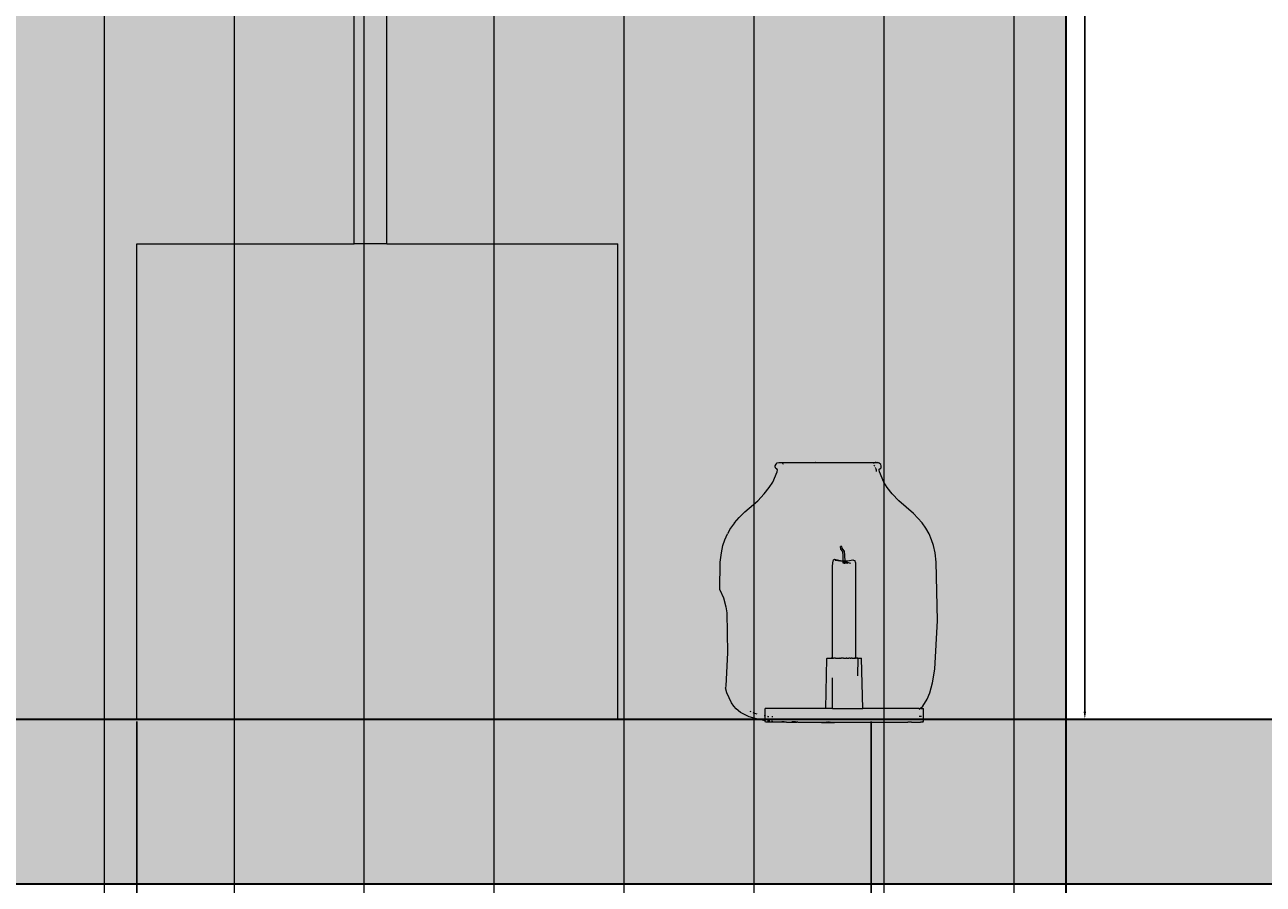
# Model space of a CAD drawing. Units: millimetres. Extents: x 446512 to 447461, y 70395 to 70610.
# Tile 35 of 39: x 447401 to 447431, y 70432 to 70453. Entities that reach past the tile are written whole.
import ezdxf

# ---------------------------------------------------------------- set-up
doc = ezdxf.new("R2010")
doc.units = ezdxf.units.MM
for name, color, linetype, lineweight in [('A-ANNO-DIMS', 2, 'Continuous', 18), ('A-FURN', 7, 'Continuous', 35), ('A-FURN-DECO', 8, 'Continuous', 13), ('A-FURN-PATT', 38, 'Continuous', 13)]:
    doc.layers.add(name, color=color, linetype=linetype, lineweight=lineweight)
doc.styles.get("Standard").update_dxf_attribs({"font": 'arial.ttf'})
doc.dimstyles.get("Standard").update_dxf_attribs({"dimtxt": 0.18, "dimasz": 0.18, "dimexe": 0.18, "dimexo": 0.0625, "dimgap": 0.09, "dimtad": 0, "dimtih": 1, "dimtoh": 1, "dimdec": 4, "dimzin": 0, "dimdsep": 46, "dimtxsty": 'Standard', "dimcen": 0.09, "dimadec": 0, "dimazin": 0, "dimtfac": 1, "dimtdec": 4, "dimtofl": 0, "dimtmove": 0, "dimatfit": 3, "dimfxl": 1, "dimtolj": 1, "dimtzin": 0, "dimarcsym": 0})

# ---------------------------------------------------------------- blocks, each defined once
blk = doc.blocks.new('DECO-SCULPTURE-BIRD')
for p, q in [((16.449, 34.749), (16.526, 34.819)), ((15.181, 34.03), (15.627, 34.749)), ((15.627, 34.749), (16.449, 34.749)), ((13.93, 33.268), (14.629, 34.03)), ((14.629, 34.03), (15.181, 34.03)), ((17.942, 33.598), (17.748, 33.234)), ((13.195, 33.309), (12.789, 32.676)), ((12.866, 33.283), (13.03, 33.299)), ((13.03, 33.299), (13.195, 33.309)), ((10.481, 32.948), (10.898, 32.983)), ((10.898, 32.983), (10.488, 31.945)), ((11.597, 32.946), (11.749, 33.008)), ((11.749, 33.008), (11.904, 33.064)), ((11.904, 33.064), (12.061, 33.115)), ((12.061, 33.115), (12.219, 33.16)), ((12.219, 33.16), (12.379, 33.199)), ((12.379, 33.199), (12.541, 33.233)), ((12.541, 33.233), (12.703, 33.261)), ((12.703, 33.261), (12.866, 33.283)), ((13.33, 33.029), (13.93, 33.268)), ((13.33, 32.676), (13.33, 33.029)), ((17.748, 33.234), (17.539, 32.879)), ((9.257, 32.674), (9.658, 32.793)), ((9.658, 32.793), (10.067, 32.884)), ((10.067, 32.884), (10.481, 32.948)), ((10.747, 31.945), (11.298, 32.806)), ((11.298, 32.806), (11.446, 32.878)), ((11.446, 32.878), (11.597, 32.946)), ((17.539, 32.879), (17.314, 32.533)), ((8.482, 32.355), (8.864, 32.528)), ((8.864, 32.528), (9.257, 32.674)), ((12.789, 32.676), (13.33, 32.676)), ((17.314, 32.533), (17.074, 32.198)), ((7.759, 31.935), (8.113, 32.157)), ((8.113, 32.157), (8.482, 32.355)), ((17.074, 32.198), (16.819, 31.874)), ((7.42, 31.689), (7.759, 31.935)), ((10.488, 31.945), (10.747, 31.945)), ((16.819, 31.874), (16.55, 31.562)), ((7.098, 31.42), (7.42, 31.689)), ((16.55, 31.562), (16.267, 31.262)), ((4.396, 31.274), (4.005, 30.703)), ((4.59, 31.141), (4.396, 31.274)), ((6.796, 31.131), (7.098, 31.42)), ((16.267, 31.262), (15.971, 30.975)), ((4.59, 31.11), (3.442, 29.152)), ((4.59, 31.141), (4.005, 30.703)), ((4.354, 30.38), (4.784, 31.008)), ((4.59, 31.11), (4.59, 31.141)), ((4.784, 31.008), (4.59, 31.141)), ((6.514, 30.821), (6.796, 31.131)), ((15.971, 30.975), (15.663, 30.701)), ((4.005, 30.703), (2.875, 29.852)), ((6.514, 30.821), (6.273, 30.344)), ((15.663, 30.701), (15.342, 30.442)), ((3.962, 29.736), (4.354, 30.38)), ((6.273, 30.344), (6.062, 29.854)), ((15.342, 30.442), (15.375, 30.385)), ((15.375, 30.385), (15.4, 30.324)), ((15.4, 30.324), (15.418, 30.261)), ((15.418, 30.261), (15.428, 30.196)), ((15.408, 30.001), (15.385, 29.939)), ((15.422, 30.065), (15.408, 30.001)), ((15.429, 30.13), (15.422, 30.065)), ((15.428, 30.196), (15.429, 30.13)), ((2.875, 29.852), (2.1, 29.278)), ((2.704, 29.597), (2.737, 29.696)), ((2.737, 29.696), (2.795, 29.783)), ((2.795, 29.783), (2.875, 29.852)), ((2.875, 29.852), (2.971, 29.899)), ((2.971, 29.899), (3.076, 29.921)), ((3.076, 29.921), (3.183, 29.915)), ((3.183, 29.915), (3.285, 29.883)), ((3.285, 29.883), (3.375, 29.827)), ((3.375, 29.827), (3.447, 29.75)), ((3.447, 29.75), (3.496, 29.657)), ((3.496, 29.657), (3.518, 29.556)), ((3.962, 29.736), (3.605, 29.071)), ((6.062, 29.854), (5.881, 29.351)), ((15.224, 29.735), (15.054, 29.609)), ((15.274, 29.778), (15.224, 29.735)), ((15.318, 29.827), (15.274, 29.778)), ((15.355, 29.881), (15.318, 29.827)), ((15.385, 29.939), (15.355, 29.881)), ((2.698, 29.494), (2.704, 29.597)), ((2.699, 29.49), (2.698, 29.494)), ((2.698, 29.476), (2.699, 29.49)), ((3.517, 29.541), (3.518, 29.556)), ((3.517, 29.541), (3.518, 29.538)), ((14.698, 29.38), (14.513, 29.277)), ((14.878, 29.491), (14.698, 29.38)), ((15.054, 29.609), (14.878, 29.491)), ((2.031, 29.139), (2.002, 28.989)), ((2.1, 29.278), (2.031, 29.139)), ((3.425, 29.125), (3.119, 28.602)), ((3.306, 29.18), (3.325, 29.171)), ((3.358, 29.194), (3.345, 29.201)), ((3.442, 29.152), (3.425, 29.125)), ((3.593, 29.046), (3.425, 29.125)), ((3.442, 29.152), (3.605, 29.071)), ((5.881, 29.351), (5.732, 28.838)), ((14.131, 29.094), (13.934, 29.015)), ((14.324, 29.181), (14.131, 29.094)), ((14.513, 29.277), (14.324, 29.181)), ((2.002, 28.958), (2.002, 28.989)), ((2.002, 28.958), (2.013, 28.805)), ((2.013, 28.805), (2.066, 28.66)), ((3.287, 28.392), (3.593, 29.046)), ((5.732, 28.838), (5.615, 28.317)), ((13.121, 28.783), (12.912, 28.746)), ((13.328, 28.828), (13.121, 28.783)), ((13.532, 28.882), (13.328, 28.828)), ((13.735, 28.944), (13.532, 28.882)), ((13.934, 29.015), (13.735, 28.944)), ((2.066, 28.66), (2.155, 28.533)), ((2.155, 28.533), (2.275, 28.433)), ((2.883, 28.399), (3.015, 28.486)), ((3.005, 28.509), (3.027, 28.499)), ((3.015, 28.486), (3.027, 28.499)), ((3.036, 28.509), (3.019, 28.518)), ((3.027, 28.499), (3.036, 28.509)), ((3.027, 28.499), (3.284, 28.387)), ((3.036, 28.509), (3.119, 28.602)), ((3.036, 28.509), (3.287, 28.392)), ((3.074, 28.492), (3.069, 28.481)), ((3.152, 28.659), (3.074, 28.492)), ((12.912, 28.746), (12.912, 28.476)), ((12.912, 28.476), (13.001, 28.48)), ((13.001, 28.48), (13.089, 28.487)), ((13.089, 28.487), (13.177, 28.496)), ((13.177, 28.496), (13.265, 28.508)), ((13.265, 28.508), (13.352, 28.523)), ((13.352, 28.523), (13.439, 28.54)), ((13.439, 28.54), (13.525, 28.559)), ((13.525, 28.559), (13.611, 28.581)), ((13.611, 28.581), (13.696, 28.606)), ((13.696, 28.606), (13.781, 28.633)), ((13.947, 28.695), (13.752, 28.315)), ((13.781, 28.633), (13.864, 28.663)), ((13.864, 28.663), (13.947, 28.695)), ((2.275, 28.433), (2.419, 28.366)), ((2.419, 28.366), (2.575, 28.337)), ((2.766, 28.36), (2.561, 27.852)), ((2.575, 28.337), (2.733, 28.349)), ((2.733, 28.349), (2.766, 28.36)), ((2.766, 28.36), (2.883, 28.399)), ((2.781, 28.395), (2.766, 28.36)), ((3.002, 27.688), (3.284, 28.387)), ((5.615, 28.317), (5.531, 27.79)), ((8.422, 28.162), (8.382, 28.133)), ((8.466, 28.185), (8.422, 28.162)), ((8.513, 28.202), (8.466, 28.185)), ((8.561, 28.212), (8.513, 28.202)), ((8.611, 28.216), (8.561, 28.212)), ((8.66, 28.212), (8.611, 28.216)), ((8.709, 28.202), (8.66, 28.212)), ((8.756, 28.185), (8.709, 28.202)), ((8.799, 28.162), (8.756, 28.185)), ((8.84, 28.133), (8.799, 28.162)), ((13.752, 28.315), (13.509, 27.964)), ((2.561, 27.852), (2.308, 27.114)), ((8.147, 27.859), (7.968, 27.605)), ((8.346, 28.098), (8.147, 27.859)), ((8.382, 28.133), (8.346, 28.098)), ((8.875, 28.098), (8.84, 28.133)), ((8.892, 27.984), (8.875, 28.098)), ((8.919, 27.871), (8.892, 27.984)), ((8.956, 27.761), (8.919, 27.871)), ((13.509, 27.964), (13.223, 27.648)), ((2.757, 26.974), (3.002, 27.688)), ((5.531, 27.79), (5.479, 27.259)), ((7.968, 27.605), (7.808, 27.338)), ((9.002, 27.655), (8.956, 27.761)), ((9.057, 27.553), (9.002, 27.655)), ((9.121, 27.456), (9.057, 27.553)), ((13.223, 27.648), (12.897, 27.372)), ((5.479, 27.259), (5.46, 26.725)), ((7.808, 27.338), (7.671, 27.059)), ((9.193, 27.366), (9.121, 27.456)), ((9.273, 27.282), (9.193, 27.366)), ((9.359, 27.205), (9.273, 27.282)), ((12.897, 27.372), (12.537, 27.142)), ((2.308, 27.114), (2.095, 26.364)), ((2.662, 26.638), (2.757, 26.974)), ((7.671, 27.059), (7.556, 26.77)), ((9.452, 27.136), (9.359, 27.205)), ((9.551, 27.075), (9.452, 27.136)), ((9.654, 27.023), (9.551, 27.075)), ((10.055, 26.875), (9.654, 27.023)), ((12.15, 26.961), (11.743, 26.833)), ((12.537, 27.142), (12.15, 26.961)), ((1.77, 26.41), (1.808, 26.703)), ((1.827, 26.703), (1.77, 26.41)), ((1.827, 26.703), (1.808, 26.703)), ((1.827, 26.703), (1.873, 26.703)), ((1.89, 26.535), (1.873, 26.703)), ((2.459, 26.45), (2.547, 26.703)), ((2.603, 26.703), (2.459, 26.45)), ((2.558, 26.703), (2.547, 26.703)), ((2.64, 26.703), (2.603, 26.703)), ((2.662, 26.638), (2.64, 26.703)), ((2.709, 26.493), (2.662, 26.638)), ((3.737, 26.466), (3.854, 26.703)), ((3.905, 26.667), (3.737, 26.466)), ((3.875, 26.703), (3.854, 26.703)), ((3.875, 26.703), (3.905, 26.667)), ((3.935, 26.703), (3.905, 26.667)), ((3.957, 26.703), (3.935, 26.703)), ((4.064, 26.48), (3.957, 26.703)), ((5.46, 26.725), (5.471, 26.308)), ((5.845, 26.703), (5.471, 26.308)), ((6.58, 25.364), (5.845, 26.703)), ((7.523, 26.665), (6.643, 25.636)), ((7.523, 26.665), (7.514, 26.636)), ((7.526, 26.673), (7.523, 26.665)), ((7.523, 26.665), (7.531, 26.655)), ((7.556, 26.77), (7.526, 26.673)), ((7.551, 26.703), (7.526, 26.673)), ((7.551, 26.703), (7.572, 26.703)), ((7.688, 26.466), (7.572, 26.703)), ((8.717, 26.493), (8.786, 26.703)), ((8.833, 26.686), (8.717, 26.493)), ((8.786, 26.703), (8.823, 26.703)), ((8.823, 26.703), (8.833, 26.686)), ((8.843, 26.703), (8.833, 26.686)), ((8.843, 26.703), (8.879, 26.703)), ((8.967, 26.45), (8.879, 26.703)), ((9.536, 26.535), (9.553, 26.703)), ((9.573, 26.703), (9.536, 26.535)), ((9.553, 26.703), (9.573, 26.703)), ((9.573, 26.703), (9.618, 26.703)), ((9.618, 26.703), (9.665, 26.337)), ((10.471, 26.78), (10.055, 26.875)), ((10.896, 26.742), (10.471, 26.78)), ((11.323, 26.759), (10.896, 26.742)), ((11.743, 26.833), (11.323, 26.759)), ((1.761, 26.337), (1.636, 25.636)), ((1.761, 26.337), (1.77, 26.41)), ((1.89, 26.535), (2.01, 25.987)), ((1.967, 25.795), (1.89, 26.535)), ((2.459, 26.45), (1.998, 25.636)), ((2.095, 26.364), (2.01, 25.987)), ((2.709, 26.493), (3.149, 25.76)), ((3.046, 25.467), (2.709, 26.493)), ((3.737, 26.466), (3.149, 25.76)), ((4.013, 26.541), (4.064, 26.48)), ((4.064, 26.48), (4.783, 25.636)), ((4.603, 25.364), (4.064, 26.48)), ((7.688, 26.466), (8.277, 25.76)), ((7.688, 26.466), (8.203, 25.423)), ((8.717, 26.493), (8.277, 25.76)), ((8.967, 26.45), (9.364, 25.75)), ((8.967, 26.45), (9.339, 25.38)), ((9.536, 26.535), (9.364, 25.75)), ((9.665, 26.337), (9.79, 25.636)), ((9.789, 25.364), (9.665, 26.337)), ((5.471, 26.308), (4.835, 25.636)), ((1.967, 25.795), (1.935, 25.655)), ((2.01, 25.987), (1.967, 25.795)), ((1.998, 25.499), (1.967, 25.795)), ((2.01, 25.987), (2.045, 25.829)), ((3.149, 25.76), (3.046, 25.636)), ((8.277, 25.76), (8.203, 25.636)), ((9.364, 25.75), (9.339, 25.636)), ((1.636, 25.636), (1.639, 25.38)), ((1.998, 25.636), (1.998, 25.499)), ((1.998, 25.499), (1.998, 24.41)), ((3.046, 25.636), (3.046, 25.467)), ((3.046, 25.467), (3.046, 24.397)), ((4.783, 25.636), (4.783, 24.41)), ((4.835, 25.636), (4.835, 24.41)), ((6.643, 25.636), (6.643, 24.617)), ((8.203, 25.636), (8.203, 25.423)), ((8.232, 25.364), (8.203, 25.423)), ((9.339, 25.636), (9.339, 25.38)), ((9.79, 25.636), (9.789, 25.364)), ((1.637, 25.364), (1.635, 24.407)), ((1.637, 25.364), (1.639, 25.38)), ((4.603, 25.364), (4.61, 24.41)), ((6.58, 25.364), (6.586, 24.617)), ((8.232, 25.364), (8.239, 24.482)), ((9.344, 25.364), (9.339, 25.38)), ((9.344, 25.364), (9.349, 24.41)), ((9.789, 25.364), (9.79, 24.407)), ((1.998, 24.556), (1.98, 24.397)), ((6.643, 24.617), (6.586, 24.617)), ((6.586, 24.617), (6.588, 24.41)), ((6.663, 24.617), (6.643, 24.617)), ((6.643, 24.617), (6.643, 24.41)), ((1.467, 24.182), (1.468, 24.235)), ((1.468, 24.235), (1.483, 24.287)), ((1.483, 24.287), (1.51, 24.333)), ((1.51, 24.333), (1.549, 24.371)), ((1.549, 24.371), (1.595, 24.397)), ((1.595, 24.397), (1.635, 24.407)), ((1.635, 24.407), (1.648, 24.41)), ((1.635, 24.407), (1.635, 24.397)), ((1.635, 24.371), (1.635, 24.182)), ((1.648, 24.41), (1.657, 24.41)), ((1.648, 24.41), (1.651, 24.41)), ((1.923, 24.41), (1.657, 24.41)), ((1.998, 24.41), (1.967, 24.41)), ((1.977, 24.371), (1.967, 24.29)), ((1.998, 24.367), (1.967, 24.367)), ((1.998, 24.41), (1.998, 24.397)), ((1.998, 24.371), (1.998, 24.367)), ((1.998, 24.367), (1.998, 24.182)), ((2.958, 24.41), (2.109, 24.41)), ((3.046, 24.371), (3.046, 24.182)), ((4.61, 24.41), (4.588, 24.41)), ((4.611, 24.367), (4.588, 24.367)), ((4.61, 24.41), (4.611, 24.397)), ((4.783, 24.41), (4.61, 24.41)), ((4.611, 24.371), (4.611, 24.367)), ((4.611, 24.367), (4.612, 24.182)), ((4.783, 24.367), (4.611, 24.367)), ((4.783, 24.41), (4.835, 24.41)), ((4.783, 24.41), (4.783, 24.397)), ((4.783, 24.371), (4.783, 24.367)), ((4.783, 24.367), (4.783, 24.182)), ((4.835, 24.367), (4.783, 24.367)), ((4.835, 24.41), (4.835, 24.397)), ((4.835, 24.371), (4.835, 24.367)), ((4.835, 24.367), (4.835, 24.182)), ((6.588, 24.41), (6.588, 24.397)), ((6.643, 24.41), (6.588, 24.41)), ((6.588, 24.371), (6.588, 24.367)), ((6.588, 24.367), (6.59, 24.182)), ((6.643, 24.367), (6.588, 24.367)), ((6.663, 24.41), (6.643, 24.41)), ((6.643, 24.41), (6.643, 24.397)), ((6.643, 24.371), (6.643, 24.367)), ((6.663, 24.367), (6.643, 24.367)), ((6.643, 24.367), (6.643, 24.182)), ((6.737, 24.41), (8.029, 24.41)), ((9.272, 24.41), (8.372, 24.41)), ((9.384, 24.41), (9.349, 24.41)), ((9.349, 24.41), (9.35, 24.397)), ((9.35, 24.371), (9.35, 24.367)), ((9.384, 24.367), (9.35, 24.367)), ((9.35, 24.367), (9.351, 24.182)), ((9.445, 24.41), (9.742, 24.41)), ((9.79, 24.407), (9.83, 24.397)), ((9.79, 24.407), (9.79, 24.397)), ((9.79, 24.371), (9.79, 24.182)), ((9.83, 24.397), (9.877, 24.371)), ((9.877, 24.371), (9.916, 24.333)), ((9.916, 24.333), (9.943, 24.287)), ((9.943, 24.287), (9.958, 24.235)), ((9.958, 24.235), (9.959, 24.182)), ((0.327, 22.505), (1.544, 24.044)), ((1.48, 24.13), (1.467, 24.182)), ((1.507, 24.083), (1.48, 24.13)), ((1.544, 24.044), (1.507, 24.083)), ((1.635, 24.13), (1.635, 24.083)), ((1.639, 24.083), (1.635, 24.083)), ((1.707, 24.083), (1.635, 24.083)), ((1.704, 24.059), (1.703, 24.044)), ((1.707, 24.083), (1.704, 24.059)), ((1.998, 24.083), (1.707, 24.083)), ((1.944, 24.083), (1.939, 24.044)), ((1.998, 24.13), (1.998, 24.083)), ((1.998, 24.083), (2.18, 24.083)), ((2.176, 24.044), (2.18, 24.083)), ((2.18, 24.083), (3.049, 24.083)), ((3.046, 24.13), (3.049, 24.083)), ((3.049, 24.083), (4.613, 24.083)), ((4.613, 24.13), (4.613, 24.083)), ((4.783, 24.083), (4.613, 24.083)), ((4.783, 24.13), (4.783, 24.083)), ((4.835, 24.13), (4.835, 24.083)), ((4.835, 24.083), (6.591, 24.083)), ((6.59, 24.13), (6.591, 24.083)), ((6.643, 24.083), (6.591, 24.083)), ((6.643, 24.13), (6.643, 24.083)), ((9.351, 24.083), (6.643, 24.083)), ((9.351, 24.13), (9.351, 24.083)), ((9.79, 24.083), (9.351, 24.083)), ((9.79, 24.13), (9.79, 24.083)), ((9.919, 24.083), (9.882, 24.044)), ((9.882, 24.044), (11.099, 22.505)), ((9.946, 24.13), (9.919, 24.083)), ((9.959, 24.182), (9.946, 24.13)), ((1.72, 20.641), (0.327, 22.505)), ((11.099, 22.505), (0.327, 22.505)), ((11.099, 22.505), (9.706, 20.641)), ((1.56, 20.562), (1.635, 20.611)), ((1.635, 20.611), (1.72, 20.641)), ((9.706, 20.641), (9.791, 20.611)), ((9.791, 20.611), (9.866, 20.562)), ((1.431, 20.239), (1.432, 20.329)), ((1.432, 20.329), (1.455, 20.417)), ((1.455, 20.417), (1.498, 20.496)), ((1.498, 20.496), (1.56, 20.562)), ((9.866, 20.562), (9.927, 20.496)), ((9.927, 20.496), (9.971, 20.417)), ((9.971, 20.417), (9.994, 20.329)), ((9.994, 20.329), (9.995, 20.239)), ((1.451, 20.152), (1.431, 20.239)), ((1.492, 20.071), (1.451, 20.152)), ((1.551, 20.003), (1.492, 20.071)), ((1.625, 19.952), (1.551, 20.003)), ((9.874, 20.003), (9.801, 19.952)), ((9.934, 20.071), (9.874, 20.003)), ((9.975, 20.152), (9.934, 20.071)), ((9.995, 20.239), (9.975, 20.152)), ((1.48, 18.035), (1.609, 19.909)), ((1.799, 19.909), (1.609, 19.909)), ((1.709, 19.92), (1.625, 19.952)), ((1.648, 18.028), (2.417, 19.746)), ((1.799, 19.909), (1.709, 19.92)), ((1.799, 19.909), (2.323, 19.909)), ((2.323, 19.909), (2.359, 19.909)), ((2.364, 19.896), (2.323, 19.909)), ((2.364, 19.896), (2.359, 19.909)), ((2.359, 19.909), (4.323, 19.909)), ((2.417, 19.746), (2.364, 19.896)), ((2.508, 19.49), (2.417, 19.746)), ((3.245, 18.169), (4.419, 19.866)), ((3.386, 17.993), (4.578, 19.714)), ((4.323, 19.909), (4.479, 19.909)), ((4.419, 19.866), (4.323, 19.909)), ((4.479, 19.866), (4.479, 19.909)), ((6.726, 19.909), (4.479, 19.909)), ((4.578, 19.714), (4.479, 19.866)), ((5.313, 18.586), (4.578, 19.714)), ((6.112, 18.612), (6.893, 19.784)), ((6.922, 19.907), (6.726, 19.909)), ((6.893, 19.784), (6.878, 19.805)), ((6.985, 19.65), (6.893, 19.784)), ((6.922, 19.907), (6.926, 19.909)), ((6.926, 19.909), (6.936, 19.909)), ((8.957, 19.909), (6.936, 19.909)), ((8.239, 18.093), (8.898, 19.762)), ((8.898, 19.762), (8.95, 19.895)), ((8.967, 19.615), (8.898, 19.762)), ((8.95, 19.895), (8.999, 19.909)), ((8.95, 19.895), (8.957, 19.909)), ((8.957, 19.909), (8.999, 19.909)), ((8.999, 19.909), (9.627, 19.909)), ((9.716, 19.92), (9.627, 19.909)), ((9.807, 19.907), (9.627, 19.909)), ((9.801, 19.952), (9.716, 19.92)), ((9.814, 19.909), (9.807, 19.907)), ((9.816, 19.893), (9.814, 19.909)), ((9.974, 18.035), (9.816, 19.893)), ((9.876, 18.035), (9.816, 19.893)), ((1.771, 17.993), (2.508, 19.49)), ((3.027, 18.035), (2.508, 19.49)), ((6.112, 18.284), (6.985, 19.65)), ((8.126, 17.993), (6.985, 19.65)), ((8.405, 18.035), (8.967, 19.615)), ((9.727, 17.993), (8.967, 19.615)), ((5.313, 11.612), (5.313, 18.586)), ((5.7, 17.993), (5.313, 18.586)), ((5.812, 18.161), (6.112, 18.612)), ((6.112, 18.612), (6.112, 18.655)), ((6.112, 18.284), (6.112, 18.612)), ((3.123, 17.993), (3.245, 18.169)), ((3.299, 18.035), (3.245, 18.169)), ((5.7, 17.993), (5.812, 18.161)), ((5.812, 18.161), (5.798, 18.182)), ((5.816, 18.155), (5.812, 18.161)), ((5.995, 18.101), (6.112, 18.284)), ((6.112, 11.612), (6.112, 18.284)), ((3.123, 17.993), (3.027, 18.035)), ((3.386, 17.993), (3.299, 18.035)), ((0, 0), (0, 11.612)), ((0, 11.612), (5.313, 11.612)), ((6.112, 11.612), (5.313, 11.612)), ((6.112, 11.612), (11.751, 11.612)), ((11.751, 0), (11.751, 11.612)), ((0, 0), (11.751, 0))]:
    blk.add_line(p, q)
blk = doc.blocks.new('*D5')
at = {"layer": 'A-ANNO-DIMS', "color": 0, "lineweight": -2, "transparency": 16777216}
for p, q in [((447421.309, 70471.106), (447426.65, 70471.106)), ((447426.47, 70470.926), (447426.47, 70453.88)), ((447426.47, 70436.468), (447426.47, 70453.514)), ((447421.309, 70436.288), (447426.65, 70436.288))]:
    blk.add_line(p, q, dxfattribs=at)
at = {"layer": 'A-ANNO-DIMS', "color": 0, "transparency": 16777216}
for points in [[(447426.44, 70470.926), (447426.5, 70470.926), (447426.47, 70471.106)], [(447426.44, 70436.468), (447426.5, 70436.468), (447426.47, 70436.288)]]:
    blk.add_solid(points, dxfattribs=at)
at = {"layer": 'Defpoints', "color": 0, "transparency": 16777216}
for p in [(447421.247, 70471.106), (447426.47, 70471.106), (447421.247, 70436.288)]:
    blk.add_point(p, dxfattribs=at)
at = {"layer": 'A-ANNO-DIMS', "color": 0, "transparency": 16777216, "insert": (447426.47, 70453.697), "char_height": 0.18, "attachment_point": 5}
blk.add_mtext('\\A1;BIRD SCULPTURE 35 TYP.', dxfattribs=at)
blk = doc.blocks.new('*D6')
at = {"layer": 'A-ANNO-DIMS', "color": 0, "lineweight": -2, "transparency": 16777216}
for p, q in [((447403.306, 70436.225), (447403.306, 70430.885)), ((447421.247, 70436.225), (447421.247, 70430.885)), ((447403.486, 70431.065), (447411.757, 70431.065)), ((447421.067, 70431.065), (447412.796, 70431.065))]:
    blk.add_line(p, q, dxfattribs=at)
at = {"layer": 'A-ANNO-DIMS', "color": 0, "transparency": 16777216}
for points in [[(447403.486, 70431.095), (447403.486, 70431.035), (447403.306, 70431.065)], [(447421.067, 70431.095), (447421.067, 70431.035), (447421.247, 70431.065)]]:
    blk.add_solid(points, dxfattribs=at)
at = {"layer": 'Defpoints', "color": 0, "transparency": 16777216}
for p in [(447403.306, 70436.288), (447421.247, 70436.288), (447421.247, 70431.065)]:
    blk.add_point(p, dxfattribs=at)
at = {"layer": 'A-ANNO-DIMS', "color": 0, "transparency": 16777216, "insert": (447412.276, 70431.065), "char_height": 0.18, "attachment_point": 5}
blk.add_mtext('\\A1;18 TYP.', dxfattribs=at)
blk = doc.blocks.new('*D61')
at = {"layer": 'A-ANNO-DIMS', "color": 0, "lineweight": -2, "transparency": 16777216}
for p, q in [((447254.943, 70452.792), (447254.943, 70394.885)), ((447450.532, 70432.19), (447450.532, 70394.885)), ((447255.123, 70395.065), (447352.352, 70395.065)), ((447450.352, 70395.065), (447353.122, 70395.065))]:
    blk.add_line(p, q, dxfattribs=at)
at = {"layer": 'A-ANNO-DIMS', "color": 0, "transparency": 16777216}
for points in [[(447255.123, 70395.095), (447255.123, 70395.035), (447254.943, 70395.065)], [(447450.352, 70395.095), (447450.352, 70395.035), (447450.532, 70395.065)]]:
    blk.add_solid(points, dxfattribs=at)
at = {"layer": 'Defpoints', "color": 0, "transparency": 16777216}
for p in [(447254.943, 70452.855), (447450.532, 70432.253), (447450.532, 70395.065)]:
    blk.add_point(p, dxfattribs=at)
at = {"layer": 'A-ANNO-DIMS', "color": 0, "transparency": 16777216, "insert": (447352.737, 70395.065), "char_height": 0.18, "attachment_point": 5}
blk.add_mtext('\\A1;195.6', dxfattribs=at)

msp = doc.modelspace()

# ---------------------------------------------------------------- hatches: boundary and pattern name
at = {"layer": 'A-FURN-PATT'}
h = msp.add_hatch(dxfattribs=at)
h.set_pattern_fill('ANSI31', color=256, angle=45)
h.set_pattern_definition([(90, (127.5626, 0), (-3.175, 0), [])])
h.paths.add_polyline_path([(447426.0142, 70599.7147), (447365.4251, 70599.7147), (447365.4251, 70405.3145), (447426.0142, 70405.3145)])
h = msp.add_hatch(color=256, dxfattribs=at)
h.dxf.hatch_style = 1
h.paths.add_polyline_path([(447426.0142, 70502.5146), (447365.4251, 70502.5146), (447365.4251, 70436.2876), (447426.0142, 70436.2876)])
h = msp.add_hatch(color=256, dxfattribs=at)
h.dxf.hatch_style = 1
h.paths.add_polyline_path([(447365.4251, 70432.2526), (447365.4251, 70436.2876), (447340.0494, 70436.2876), (447340.0494, 70432.2526)])
h.paths.add_polyline_path([(447426.0142, 70436.2876), (447426.0142, 70432.2526), (447450.5318, 70432.2526), (447450.5318, 70436.2876)])
h = msp.add_hatch(color=256, dxfattribs=at)
h.dxf.hatch_style = 1
h.paths.add_polyline_path([(447426.0142, 70432.2526), (447426.0142, 70436.2876), (447365.4251, 70436.2876), (447365.4251, 70432.2526)])
h = msp.add_hatch(color=256, dxfattribs=at)
h.dxf.hatch_style = 1
h.paths.add_polyline_path([(447426.0142, 70432.2526), (447426.0142, 70436.2876), (447365.4251, 70436.2876), (447365.4251, 70432.2526)])
h = msp.add_hatch(color=256, dxfattribs=at)
h.dxf.hatch_style = 1
h.paths.add_polyline_path([(447426.0142, 70432.2526), (447426.0142, 70436.2876), (447365.4251, 70436.2876), (447365.4251, 70432.2526)])

# ---------------------------------------------------------------- linework, layer by layer
at = {"layer": 'A-FURN'}
msp.add_line((447426.0142, 70405.3145), (447426.0142, 70599.7147), dxfattribs=at)
msp.add_lwpolyline([(447340.0494, 70436.2876), (447450.5318, 70436.2876), (447450.5318, 70432.2526), (447340.0494, 70432.2526)], close=True, dxfattribs=at)
at = {"layer": 'A-FURN-DECO'}
for p, q in [((447418.8426, 70442.0774), (447418.9509, 70442.3274)), ((447418.9032, 70442.4408), (447418.9074, 70442.4763)), ((447418.9032, 70442.4408), (447418.9128, 70442.4198)), ((447418.9074, 70442.4763), (447418.927, 70442.5163)), ((447418.9435, 70442.4028), (447418.9128, 70442.4198)), ((447418.927, 70442.5163), (447418.9563, 70442.5445)), ((447418.9591, 70442.3808), (447418.9435, 70442.4028)), ((447418.9509, 70442.3274), (447418.9591, 70442.3808)), ((447418.9563, 70442.5445), (447418.9903, 70442.5591)), ((447418.9903, 70442.5591), (447419.0659, 70442.5532)), ((447418.9903, 70442.5591), (447419.8822, 70442.5591)), ((447419.0659, 70442.5532), (447419.0937, 70442.5304)), ((447419.0937, 70442.5304), (447419.0959, 70442.5172)), ((447419.8916, 70442.5587), (447419.8822, 70442.5591)), ((447419.8916, 70442.5587), (447421.3678, 70442.5591)), ((447421.3032, 70442.5549), (447421.3509, 70442.5566)), ((447421.3207, 70442.5463), (447421.3075, 70442.5311)), ((447421.3152, 70442.4901), (447421.334, 70442.4759)), ((447421.3509, 70442.5566), (447421.3207, 70442.5463)), ((447421.334, 70442.4759), (447421.3385, 70442.463)), ((447421.3495, 70442.4316), (447421.3519, 70442.4249)), ((447421.3678, 70442.5591), (447421.3509, 70442.5566)), ((447421.3555, 70442.4146), (447421.3686, 70442.3771)), ((447421.3705, 70442.5591), (447421.3678, 70442.5591)), ((447421.3686, 70442.3771), (447421.3752, 70442.339)), ((447421.3705, 70442.5591), (447421.4124, 70442.5587)), ((447421.447, 70442.5429), (447421.4124, 70442.5587)), ((447421.4416, 70442.3808), (447421.4472, 70442.3927)), ((447421.4498, 70442.3274), (447421.4416, 70442.3808)), ((447421.4816, 70442.5036), (447421.447, 70442.5429)), ((447421.4472, 70442.3927), (447421.486, 70442.4182)), ((447421.5581, 70442.0774), (447421.4498, 70442.3274)), ((447421.4933, 70442.4763), (447421.4816, 70442.5036)), ((447421.486, 70442.4182), (447421.4965, 70442.4353)), ((447421.4965, 70442.4353), (447421.4933, 70442.4763)), ((447418.7566, 70441.9444), (447418.8426, 70442.0774)), ((447421.6441, 70441.9444), (447421.5581, 70442.0774)), ((447418.4766, 70441.6225), (447418.6365, 70441.7917)), ((447418.6365, 70441.7917), (447418.7566, 70441.9444)), ((447421.7642, 70441.7917), (447421.6441, 70441.9444)), ((447421.9241, 70441.6225), (447421.7642, 70441.7917)), ((447418.1645, 70441.3518), (447418.4766, 70441.6225)), ((447422.2811, 70441.3129), (447421.9241, 70441.6225)), ((447417.906, 70441.0833), (447418.02, 70441.2155)), ((447418.02, 70441.2155), (447418.1196, 70441.3129)), ((447418.1196, 70441.3129), (447418.1645, 70441.3518)), ((447422.4947, 70441.0833), (447422.2811, 70441.3129)), ((447417.675, 70440.6704), (447417.7353, 70440.8106)), ((447417.8117, 70440.9483), (447417.7353, 70440.8106)), ((447417.906, 70441.0833), (447417.8117, 70440.9483)), ((447422.589, 70440.9483), (447422.4947, 70441.0833)), ((447422.6654, 70440.8106), (447422.589, 70440.9483)), ((447422.7257, 70440.6704), (447422.6654, 70440.8106)), ((447417.5885, 70440.3458), (447417.6289, 70440.5276)), ((447417.6289, 70440.5276), (447417.675, 70440.6704)), ((447420.5309, 70440.5051), (447420.4996, 70440.5034)), ((447420.5074, 70440.4417), (447420.4996, 70440.5034)), ((447420.5382, 70440.4626), (447420.5309, 70440.5051)), ((447422.7718, 70440.5276), (447422.7257, 70440.6704)), ((447422.8122, 70440.3458), (447422.7718, 70440.5276)), ((447417.5604, 70440.1229), (447417.5885, 70440.3458)), ((447420.5602, 70440.3834), (447420.5074, 70440.4417)), ((447420.5875, 70440.3967), (447420.5382, 70440.4626)), ((447420.5624, 70440.2777), (447420.5602, 70440.3834)), ((447420.5656, 70440.1565), (447420.5624, 70440.2777)), ((447420.5875, 70440.3967), (447420.6036, 70440.1564)), ((447422.8403, 70440.1229), (447422.8122, 70440.3458)), ((447417.5477, 70439.4421), (447417.5604, 70440.1229)), ((447420.3018, 70440.0236), (447420.3177, 70440.1645)), ((447420.3018, 70437.7756), (447420.3018, 70440.0236)), ((447420.3564, 70440.1825), (447420.3177, 70440.1645)), ((447420.4964, 70440.1566), (447420.3564, 70440.1825)), ((447420.4685, 70440.1418), (447420.3693, 70440.1728)), ((447420.3693, 70440.1728), (447420.4964, 70440.1566)), ((447420.4964, 70440.1566), (447420.5656, 70440.1565)), ((447420.5661, 70440.138), (447420.4964, 70440.1566)), ((447420.5669, 70440.111), (447420.5475, 70440.117)), ((447420.5661, 70440.138), (447420.5656, 70440.1565)), ((447420.5656, 70440.1565), (447420.6036, 70440.1564)), ((447420.6056, 70440.1279), (447420.5661, 70440.138)), ((447420.5663, 70440.1319), (447420.5662, 70440.1355)), ((447420.5669, 70440.111), (447420.5665, 70440.1232)), ((447420.5863, 70440.1049), (447420.5669, 70440.111)), ((447420.5672, 70440.0972), (447420.5669, 70440.111)), ((447420.5923, 70440.0959), (447420.5672, 70440.0972)), ((447420.5863, 70440.1049), (447420.6072, 70440.1031)), ((447420.5923, 70440.0959), (447420.6077, 70440.0955)), ((447420.6036, 70440.1564), (447420.6056, 70440.1279)), ((447420.6036, 70440.1564), (447420.6762, 70440.1563)), ((447420.7489, 70440.0912), (447420.6056, 70440.1279)), ((447420.6059, 70440.1229), (447420.6067, 70440.1102)), ((447420.6072, 70440.1031), (447420.6077, 70440.0955)), ((447420.6072, 70440.1031), (447420.6805, 70440.0969)), ((447420.6762, 70440.1563), (447420.8033, 70440.1755)), ((447420.8033, 70440.1755), (447420.8549, 70440.1558)), ((447420.8668, 70440.11), (447420.8549, 70440.1558)), ((447420.8668, 70440.11), (447420.8694, 70437.7756)), ((447422.8663, 70438.6926), (447422.8403, 70440.1229)), ((447417.5477, 70439.4421), (447417.6408, 70439.2528)), ((447417.6408, 70439.2528), (447417.6997, 70439.0317)), ((447417.6997, 70439.0317), (447417.7189, 70438.8799)), ((447417.7189, 70438.8799), (447417.7366, 70437.9058)), ((447422.8063, 70437.509), (447422.8663, 70438.6926)), ((447417.7366, 70437.9058), (447417.6957, 70437.0996)), ((447420.1402, 70436.5457), (447420.1684, 70437.7714)), ((447420.1684, 70437.7714), (447420.1735, 70437.7756)), ((447420.1735, 70437.7756), (447420.21, 70437.7756)), ((447420.21, 70437.7756), (447420.2121, 70437.7756)), ((447420.2121, 70437.7756), (447420.2284, 70437.7756)), ((447420.2284, 70437.7756), (447420.2321, 70437.7756)), ((447420.2321, 70437.7756), (447420.2337, 70437.7756)), ((447420.2337, 70437.7756), (447420.2448, 70437.7756)), ((447420.2448, 70437.7756), (447420.2505, 70437.7756)), ((447420.2505, 70437.7756), (447420.2539, 70437.7756)), ((447420.2539, 70437.7756), (447420.2558, 70437.7756)), ((447420.2558, 70437.7756), (447420.2584, 70437.7756)), ((447420.2584, 70437.7756), (447420.2626, 70437.7757)), ((447420.2654, 70437.7757), (447420.2626, 70437.7757)), ((447420.2626, 70437.7757), (447420.2626, 70437.7714)), ((447420.2654, 70437.7757), (447420.2673, 70437.7756)), ((447420.2673, 70437.7756), (447420.2724, 70437.7757)), ((447420.2809, 70437.7757), (447420.2724, 70437.7757)), ((447420.2831, 70437.7756), (447420.2809, 70437.7757)), ((447420.2831, 70437.7756), (447420.2909, 70437.7756)), ((447420.2909, 70437.7756), (447420.2931, 70437.7757)), ((447420.2931, 70437.7757), (447420.2944, 70437.7757)), ((447420.2944, 70437.7757), (447420.3018, 70437.7756)), ((447420.3018, 70437.7714), (447420.3018, 70437.7756)), ((447420.3123, 70437.7756), (447420.3018, 70437.7756)), ((447420.3123, 70437.7756), (447420.3257, 70437.7757)), ((447420.3716, 70437.7757), (447420.3257, 70437.7757)), ((447420.3786, 70437.7756), (447420.3716, 70437.7757)), ((447420.3786, 70437.7756), (447420.415, 70437.7756)), ((447420.415, 70437.7756), (447420.4238, 70437.7757)), ((447420.4238, 70437.7757), (447420.4824, 70437.7757)), ((447420.4926, 70437.7756), (447420.4824, 70437.7757)), ((447420.4926, 70437.7756), (447420.5134, 70437.7757)), ((447420.574, 70437.7756), (447420.5134, 70437.7757)), ((447420.574, 70437.7756), (447420.5775, 70437.7757)), ((447420.5775, 70437.7757), (447420.6421, 70437.7757)), ((447420.6561, 70437.7756), (447420.6421, 70437.7757)), ((447420.6561, 70437.7756), (447420.6964, 70437.7756)), ((447420.6964, 70437.7756), (447420.7048, 70437.7757)), ((447420.7283, 70437.7756), (447420.7048, 70437.7757)), ((447420.7311, 70437.7756), (447420.7283, 70437.7756)), ((447420.7346, 70437.7757), (447420.7311, 70437.7756)), ((447420.7346, 70437.7757), (447420.7372, 70437.7756)), ((447420.7372, 70437.7756), (447420.7389, 70437.7756)), ((447420.7389, 70437.7756), (447420.7605, 70437.7757)), ((447420.7692, 70437.7756), (447420.7605, 70437.7757)), ((447420.7864, 70437.7756), (447420.7692, 70437.7756)), ((447420.7864, 70437.7756), (447420.79, 70437.7757)), ((447420.79, 70437.7757), (447420.8377, 70437.7757)), ((447420.8439, 70437.7756), (447420.8377, 70437.7757)), ((447420.8439, 70437.7756), (447420.8612, 70437.7756)), ((447420.8657, 70437.7756), (447420.8612, 70437.7756)), ((447420.8694, 70437.7756), (447420.8657, 70437.7756)), ((447420.8694, 70437.7756), (447420.8694, 70437.7714)), ((447420.8707, 70437.7756), (447420.8694, 70437.7756)), ((447420.8744, 70437.7757), (447420.8707, 70437.7756)), ((447420.876, 70437.7757), (447420.8744, 70437.7757)), ((447420.876, 70437.7757), (447420.8855, 70437.7756)), ((447420.8886, 70437.7756), (447420.8855, 70437.7756)), ((447420.9012, 70437.7756), (447420.8886, 70437.7756)), ((447420.9044, 70437.7756), (447420.9012, 70437.7756)), ((447420.9044, 70437.7756), (447420.9127, 70437.7757)), ((447420.9219, 70437.7757), (447420.9127, 70437.7757)), ((447420.9219, 70437.7757), (447420.9155, 70437.3413)), ((447420.9247, 70437.7756), (447420.9219, 70437.7757)), ((447420.9275, 70437.7756), (447420.9247, 70437.7756)), ((447420.9275, 70437.7756), (447420.9451, 70437.7756)), ((447420.9451, 70437.7756), (447420.949, 70437.7756)), ((447420.949, 70437.7756), (447420.953, 70437.7756)), ((447420.953, 70437.7756), (447420.9676, 70437.7756)), ((447420.9676, 70437.7756), (447420.9702, 70437.7756)), ((447420.9702, 70437.7756), (447420.9722, 70437.7756)), ((447420.9722, 70437.7756), (447420.9787, 70437.7756)), ((447420.9787, 70437.7756), (447421.0111, 70437.7756)), ((447421.0159, 70437.7714), (447421.0111, 70437.7756)), ((447421.0441, 70436.5457), (447421.0159, 70437.7714)), ((447422.7466, 70437.1711), (447422.8063, 70437.509)), ((447420.3018, 70436.5457), (447420.3018, 70437.2966)), ((447422.6788, 70436.9311), (447422.7466, 70437.1711)), ((447417.6957, 70437.0996), (447417.6875, 70437.0529)), ((447417.7219, 70436.9311), (447417.6875, 70437.0529)), ((447417.836, 70436.6825), (447417.7219, 70436.9311)), ((447422.6145, 70436.7742), (447422.6788, 70436.9311)), ((447417.8918, 70436.6025), (447417.836, 70436.6825)), ((447417.9538, 70436.535), (447417.8918, 70436.6025)), ((447422.4487, 70436.5456), (447422.5089, 70436.6025)), ((447422.5089, 70436.6025), (447422.6145, 70436.7742)), ((447418.0604, 70436.4518), (447417.9538, 70436.535)), ((447418.1402, 70436.4048), (447418.0604, 70436.4518)), ((447418.2715, 70436.3459), (447418.1402, 70436.4048)), ((447418.4148, 70436.2997), (447418.2715, 70436.3459)), ((447418.2883, 70436.4778), (447418.3075, 70436.4701)), ((447418.3572, 70436.4501), (447418.3967, 70436.4342)), ((447418.3967, 70436.4342), (447418.4589, 70436.4163)), ((447418.6206, 70436.2554), (447418.4148, 70436.2997)), ((447418.6553, 70436.2513), (447418.6206, 70436.2554)), ((447418.6377, 70436.3744), (447418.6555, 70436.371)), ((447418.6553, 70436.2513), (447418.6555, 70436.371)), ((447418.6555, 70436.371), (447418.6558, 70436.5457)), ((447418.6555, 70436.371), (447418.6687, 70436.3685)), ((447420.1402, 70436.5457), (447418.6558, 70436.5457)), ((447418.7163, 70436.3594), (447418.7446, 70436.3541)), ((447418.7163, 70436.3496), (447418.7252, 70436.3496)), ((447418.7252, 70436.3496), (447418.7519, 70436.3494)), ((447418.7446, 70436.3541), (447418.7511, 70436.3538)), ((447418.8192, 70436.3514), (447418.8475, 70436.3504)), ((447418.8198, 70436.3489), (447418.8475, 70436.3488)), ((447420.3018, 70436.5457), (447420.1402, 70436.5457)), ((447420.3018, 70436.5457), (447421.0441, 70436.5457)), ((447422.4225, 70436.5457), (447421.0441, 70436.5457)), ((447422.4225, 70436.5457), (447422.4487, 70436.5456)), ((447422.4225, 70436.5204), (447422.4487, 70436.5456)), ((447422.459, 70436.3496), (447422.4228, 70436.3493)), ((447422.457, 70436.5456), (447422.4487, 70436.5456)), ((447422.4677, 70436.5457), (447422.457, 70436.5456)), ((447422.4764, 70436.3496), (447422.459, 70436.3496)), ((447422.4677, 70436.5457), (447422.5285, 70436.5457)), ((447422.529, 70436.2325), (447422.5285, 70436.5457)), ((447418.6553, 70436.2325), (447418.6553, 70436.2513)), ((447418.6774, 70436.2487), (447418.6553, 70436.2513)), ((447418.6701, 70436.2148), (447418.6553, 70436.2325)), ((447419.1554, 70436.2148), (447418.6701, 70436.2148)), ((447418.7729, 70436.2373), (447418.7161, 70436.2441)), ((447418.8506, 70436.2281), (447418.8138, 70436.2325)), ((447419.0522, 70436.2225), (447419.0665, 70436.223)), ((447419.072, 70436.223), (447419.0665, 70436.223)), ((447419.1185, 70436.2228), (447419.072, 70436.223)), ((447419.1223, 70436.2223), (447419.1185, 70436.2228)), ((447419.1709, 70436.2158), (447419.1554, 70436.2148)), ((447419.1784, 70436.2148), (447419.1709, 70436.2158)), ((447419.1784, 70436.2148), (447419.4326, 70436.2148)), ((447419.3984, 70436.2217), (447419.309, 70436.2221)), ((447419.4326, 70436.2148), (447419.3124, 70436.2159)), ((447419.4014, 70436.2214), (447419.3984, 70436.2217)), ((447419.4457, 70436.2164), (447419.4326, 70436.2148)), ((447419.46, 70436.2148), (447419.4457, 70436.2164)), ((447419.46, 70436.2148), (447420.1482, 70436.2148)), ((447420.0387, 70436.2009), (447420.1545, 70436.2128)), ((447420.0387, 70436.2009), (447420.3562, 70436.2009)), ((447420.1545, 70436.2128), (447420.1482, 70436.2148)), ((447420.1545, 70436.2128), (447420.1859, 70436.2148)), ((447420.2181, 70436.2128), (447420.1859, 70436.2148)), ((447420.2307, 70436.2148), (447420.2181, 70436.2128)), ((447420.2307, 70436.2148), (447420.2639, 70436.2128)), ((447420.2639, 70436.2128), (447420.278, 70436.2148)), ((447420.3562, 70436.2009), (447420.2639, 70436.2128)), ((447420.278, 70436.2148), (447422.0288, 70436.2148)), ((447422.0288, 70436.2148), (447422.1478, 70436.2155)), ((447422.2332, 70436.2148), (447422.1478, 70436.2155)), ((447422.2332, 70436.2148), (447422.2484, 70436.2152)), ((447422.2484, 70436.2152), (447422.2497, 70436.215)), ((447422.2484, 70436.2152), (447422.2511, 70436.2152)), ((447422.2511, 70436.2152), (447422.3237, 70436.2148)), ((447422.3237, 70436.2148), (447422.3372, 70436.215)), ((447422.3372, 70436.215), (447422.3385, 70436.215)), ((447422.3385, 70436.215), (447422.3975, 70436.2148)), ((447422.3975, 70436.2148), (447422.4378, 70436.2148)), ((447422.4378, 70436.2148), (447422.4539, 70436.2148)), ((447422.4622, 70436.2149), (447422.4539, 70436.2148)), ((447422.5142, 70436.2148), (447422.4622, 70436.2149)), ((447422.5142, 70436.2148), (447422.529, 70436.2325))]:
    msp.add_line(p, q, dxfattribs=at)

# ---------------------------------------------------------------- block references
msp.add_blockref('DECO-SCULPTURE-BIRD', (447403.3053, 70436.2876), dxfattribs=at)

# ---------------------------------------------------------------- dimensions: what is measured, and where the dimension line sits
at = {"layer": 'A-ANNO-DIMS'}
dim = msp.add_linear_dim(base=(447426.4697, 70471.1062), p1=(447421.2469, 70436.2876), p2=(447421.2469, 70471.1062), angle=90, text='BIRD SCULPTURE <> TYP.', dimstyle='Standard', override={"dimdec": 0, "dimlfac": 1, "dimrnd": 0, "dimzin": 0, "dimdsep": 46, "dimlunit": 2}, dxfattribs=at)
dim.commit()
dim.dimension.update_dxf_attribs({"geometry": '*D5', "text_midpoint": (447426.4697, 70453.6969)})
dim = msp.add_linear_dim(base=(447450.5318, 70395.0645), p1=(447254.9427, 70452.855), p2=(447450.5318, 70432.2526), dimstyle='Standard', override={"dimdec": 1, "dimlfac": 1, "dimrnd": 0, "dimzin": 0, "dimdsep": 46, "dimlunit": 2}, dxfattribs=at)
dim.commit()
dim.dimension.update_dxf_attribs({"geometry": '*D61', "text_midpoint": (447352.7372, 70395.0645)})
dim = msp.add_linear_dim(base=(447421.2469, 70431.0648), p1=(447403.3055, 70436.2876), p2=(447421.2469, 70436.2876), text='<> TYP.', dimstyle='Standard', override={"dimdec": 0, "dimlfac": 1, "dimrnd": 0, "dimzin": 0, "dimdsep": 46, "dimlunit": 2}, dxfattribs=at)
dim.commit()
dim.dimension.update_dxf_attribs({"geometry": '*D6', "text_midpoint": (447412.2762, 70431.0648)})

doc.saveas('drawing.dxf')
